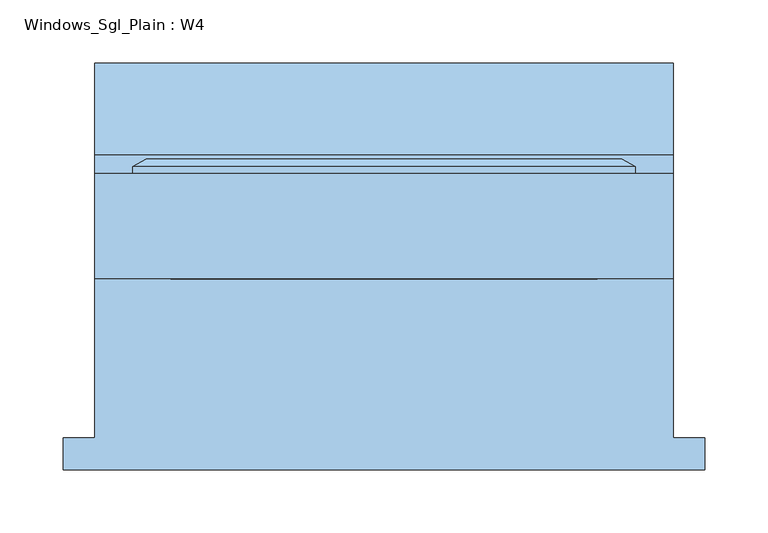
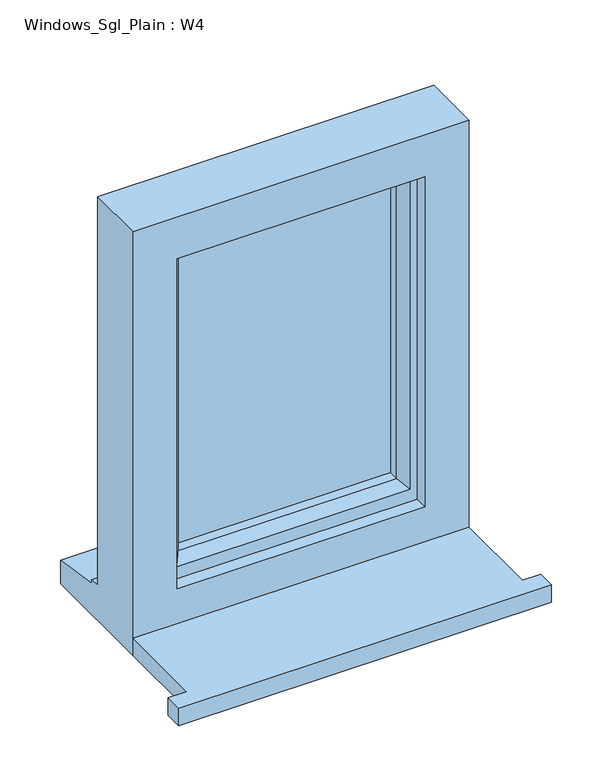
"""IFC4 building model written with IfcOpenShell, lengths in millimetres: window geometry, Windows_Sgl_Plain : W4."""

from ifc_helpers import new_model, si_unit, frame, origin, place, context, project, spatial, polyline, outline, extrude, faceted_brep, source, transform, mapped, element, save


def windows_sgl_plain_w4_7e877f05(model_context):
    return source(origin(), model_context, "Body", "SolidModel", [
        extrude(outline(polyline([(-253.6, -146.0834322), (-253.6, -121.0834322), (-228.6, -121.0834322), (-228.6, 4.9965678), (228.6, 4.9965678), (228.6, -121.0834322), (253.6, -121.0834322), (253.6, -146.0834322), (-253.6, -146.0834322)])), frame((0.0, 0.0, 1500.4), z_axis=(0.0, 0.0, 1.0), x_axis=(1.0, 0.0, 0.0)), (0.0, 0.0, 1.0), 25.0),
        faceted_brep([(-228.6, 4.9965678, 1500.4), (228.6, 4.9965678, 1500.4), (228.6, 4.9965678, 2110.0), (-228.6, 4.9965678, 2110.0), (-168.6, 4.9965678, 2050.0), (168.6, 4.9965678, 2050.0), (168.6, 4.9965678, 1575.4), (-168.6, 4.9965678, 1575.4), (-228.6, 87.9965678, 2110.0), (-228.6, 87.9965678, 1551.4), (-228.6, 102.9965678, 1550.08767), (-228.6, 102.9965678, 1545.1449676), (-228.6, 175.4965678, 1534.2088847), (-228.6, 175.4965678, 1500.4), (228.6, 87.9965678, 2110.0), (228.6, 87.9965678, 1551.4), (-188.6, 87.9965678, 2070.0), (-188.6, 87.9965678, 1563.4), (188.6, 87.9965678, 1563.4), (188.6, 87.9965678, 2070.0), (-188.6, 22.9965678, 2070.0), (-188.6, 22.9965678, 1563.4), (188.6, 22.9965678, 2070.0), (188.6, 22.9965678, 1563.4), (-168.6, 22.9965678, 2050.0), (-168.6, 22.9965678, 1575.4), (168.6, 22.9965678, 1575.4), (168.6, 22.9965678, 2050.0), (228.6, 175.4965678, 1500.4), (228.6, 175.4965678, 1534.2088847), (228.6, 102.9965678, 1545.1449676), (228.6, 102.9965678, 1550.08767)], [[[0, 1, 2, 3], [4, 5, 6, 7]], [[0, 3, 8, 9, 10, 11, 12, 13]], [[9, 8, 14, 15], [16, 17, 18, 19]], [[17, 16, 20, 21]], [[20, 22, 23, 21], [24, 25, 26, 27]], [[24, 4, 7, 25]], [[3, 2, 14, 8]], [[16, 19, 22, 20]], [[5, 4, 24, 27]], [[15, 14, 2, 1, 28, 29, 30, 31]], [[19, 18, 23, 22]], [[5, 27, 26, 6]], [[28, 1, 0, 13]], [[29, 28, 13, 12]], [[30, 29, 12, 11]], [[31, 30, 11, 10]], [[15, 31, 10, 9]], [[21, 23, 18, 17]], [[7, 6, 26, 25]]]),
        extrude(outline(polyline([(158.6, 51.9965678), (-158.6, 51.9965678), (-158.6, 75.9965678), (158.6, 75.9965678), (158.6, 51.9965678)])), frame((0.0, 0.0, 1593.4), z_axis=(0.0, 0.0, 1.0), x_axis=(1.0, 0.0, 0.0)), (0.0, 0.0, 1.0), 446.6),
        faceted_brep([(-198.6, 87.9965678, 2080.0), (-198.6, 93.7700705, 2080.0), (-198.6, 93.7700705, 1553.4), (-198.6, 87.9965678, 1553.4), (-188.6, 22.9965678, 2070.0), (-188.6, 87.9965678, 2070.0), (-188.6, 87.9965678, 1563.4), (-188.6, 22.9965678, 1563.4), (-148.6, 37.4894677, 2030.0), (-158.7480377, 22.9965678, 2040.1480377), (-158.7480377, 22.9965678, 1593.2519623), (-148.6, 37.4894677, 1603.4), (-148.6, 51.9965678, 2030.0), (-148.6, 51.9965678, 1603.4), (-158.6, 75.9965678, 2040.0), (-158.6, 51.9965678, 2040.0), (-158.6, 51.9965678, 1593.4), (-158.6, 75.9965678, 1593.4), (-148.6, 93.7700705, 2030.0), (-148.6, 75.9965678, 2030.0), (-148.6, 75.9965678, 1603.4), (-148.6, 93.7700705, 1603.4), (-166.0457548, 99.5435732, 2047.4457548), (-166.0457548, 99.5435732, 1585.9542452), (-187.8153903, 99.5435732, 2069.2153903), (-187.8153903, 99.5435732, 1564.1846097), (198.6, 93.7700705, 1553.4), (198.6, 87.9965678, 1553.4), (188.6, 87.9965678, 1563.4), (188.6, 22.9965678, 1563.4), (158.7480377, 22.9965678, 1593.2519623), (148.6, 37.4894677, 1603.4), (148.6, 51.9965678, 1603.4), (158.6, 51.9965678, 1593.4), (158.6, 75.9965678, 1593.4), (148.6, 75.9965678, 1603.4), (148.6, 93.7700705, 1603.4), (166.0457548, 99.5435732, 1585.9542452), (187.8153903, 99.5435732, 1564.1846097), (198.6, 93.7700705, 2080.0), (198.6, 87.9965678, 2080.0), (188.6, 87.9965678, 2070.0), (188.6, 22.9965678, 2070.0), (158.7480377, 22.9965678, 2040.1480377), (148.6, 37.4894677, 2030.0), (148.6, 51.9965678, 2030.0), (158.6, 51.9965678, 2040.0), (158.6, 75.9965678, 2040.0), (148.6, 75.9965678, 2030.0), (148.6, 93.7700705, 2030.0), (166.0457548, 99.5435732, 2047.4457548), (187.8153903, 99.5435732, 2069.2153903)], [[[0, 1, 2, 3]], [[4, 5, 6, 7]], [[8, 9, 10, 11]], [[12, 8, 11, 13]], [[14, 15, 16, 17]], [[18, 19, 20, 21]], [[22, 18, 21, 23]], [[1, 24, 25, 2]], [[3, 2, 26, 27]], [[7, 6, 28, 29]], [[11, 10, 30, 31]], [[13, 11, 31, 32]], [[17, 16, 33, 34]], [[21, 20, 35, 36]], [[23, 21, 36, 37]], [[2, 25, 38, 26]], [[27, 26, 39, 40]], [[29, 28, 41, 42]], [[31, 30, 43, 44]], [[32, 31, 44, 45]], [[34, 33, 46, 47]], [[36, 35, 48, 49]], [[37, 36, 49, 50]], [[26, 38, 51, 39]], [[40, 39, 1, 0]], [[3, 27, 40, 0], [5, 41, 28, 6]], [[42, 41, 5, 4]], [[7, 29, 42, 4], [9, 43, 30, 10]], [[44, 43, 9, 8]], [[45, 44, 8, 12]], [[15, 46, 33, 16], [13, 32, 45, 12]], [[47, 46, 15, 14]], [[17, 34, 47, 14], [19, 48, 35, 20]], [[49, 48, 19, 18]], [[50, 49, 18, 22]], [[24, 51, 38, 25], [23, 37, 50, 22]], [[39, 51, 24, 1]]]),
    ])


if __name__ == "__main__":
    model = new_model("IFC4")
    model_context = context("Model", 3, world=origin())
    ifc_project = project(units=[si_unit("LENGTHUNIT", "METRE", prefix="MILLI")], contexts=[model_context])
    site = spatial("IfcSite", under=ifc_project)
    building = spatial("IfcBuilding", under=site)
    placement = place(None, origin())
    windows_sgl_plain_w4_shape = windows_sgl_plain_w4_7e877f05(model_context)
    element("IfcWindow", 1, ObjectType="Windows_Sgl_Plain : W4", at=placement, inside=building, context=model_context, shape_type="MappedRepresentation", body=[
        mapped(windows_sgl_plain_w4_shape, transform((0.0, 0.0, 0.0), x_axis=(1.0, 0.0, 0.0), y_axis=(0.0, 1.0, 0.0), z_axis=(0.0, 0.0, 1.0))),
    ])
    save(model, "model.ifc")

# Revit data of these elements
# Type "Windows_Sgl_Plain : W4"
#   Type Mark = "59"
#   Operation = "SinglePanel"
#   Construction Type Id = "SGL"
#   Manufacturer = "Revit"
#   Keynote = "L10"
#   Analytic Construction = "Large single-glazed windows"
#   Wrap Layers (Ext) from Ext = 0.336286 ft
#   Wrap Layers (Int) from Ext = 0.582349 ft
#   Window Board Projection = 0.082021 ft
#   Window Board Extension = 0.082021 ft
#   Visual Light Transmittance = 0.9
#   Solar Heat Gain Coefficient = 0.86
#   Rough Width = 1.5 ft
#   Rough Height = 2.0 ft
#   Height = 2.0 ft
#   Width = 1.5 ft
#   Heat Transfer Coefficient (U) = 5.5617 W/(m²·K)
#   Glazing Thickness = 0.07874 ft
#   FrameOffset - External = 0.164042 ft
#   Frame Depth = 0.213255 ft
#   Default Head Height = 6.922572 ft
#   Cill Depth = 0.287073 ft
#   Cavity Closer Width = 0.164042 ft
#   Cavity Closer Offset from Ext = 0.336286 ft
#   Cavity Closer Depth = 0.278871 ft
#   Vis - Cavity Closers = yes
#   Define Thermal Properties by = 1
#   Material Trim = Window Frame
#   Material Glass = Glass
#   Material Frame = Window Frame
#   Wall Closure = (empty or 0)
# Element 1 (IfcWindow, "Windows_Sgl_Plain : W4")
#   Materials on its faces: "Window Frame", "Glass"
# Materials
#   "Window Frame": colour RGB 249 249 249, transparency 0, Keynote = "L10", Cost = 0
#   "Glass": class "Glass", colour RGB 0 128 192, transparency 0.9, Description = "Soda Lime Glass", Cost = 0
